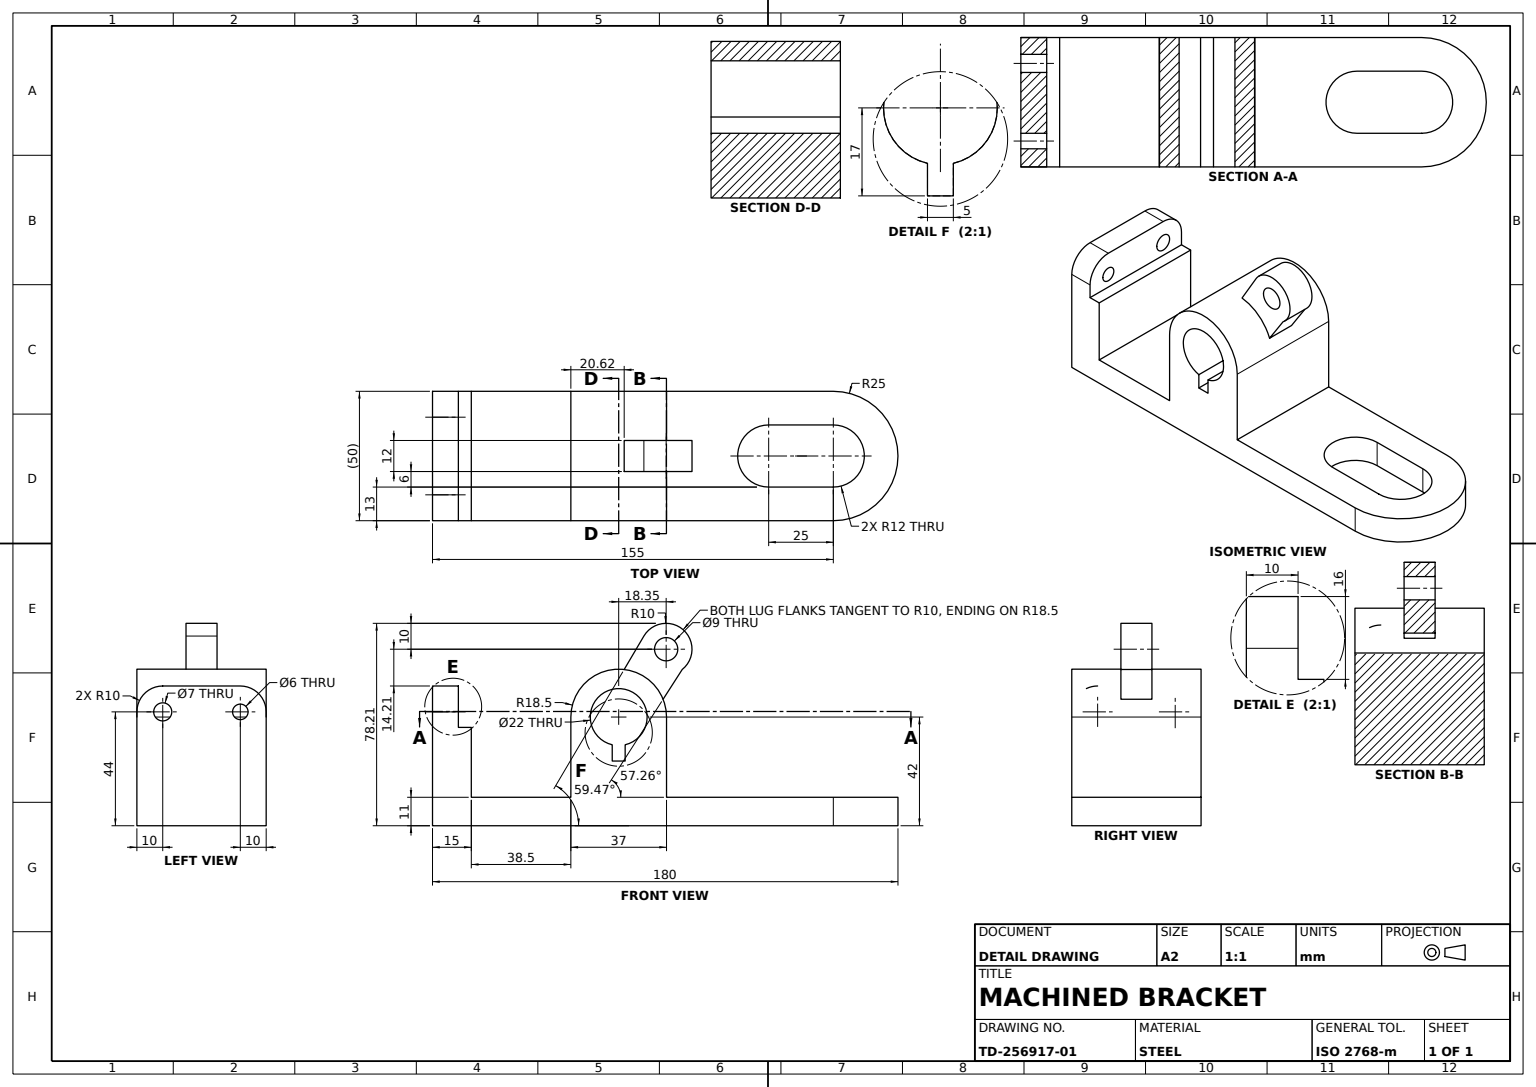
SolidWorks part; units mm, degrees
material "Plain Carbon Steel"
ref_plane "Front Plane" through (0, 0, 0) normal (0, 0, 1) x (1, 0, 0)
ref_plane "Top Plane" through (0, 0, 0) normal (0, 1, 0) x (1, 0, 0)
ref_plane "Right Plane" through (0, 0, 0) normal (1, 0, 0) x (0, 0, -1)
sketch "Base Plate Sketch" plane through (0, 0, 0) normal (0, 1, 0) x (1, 0, 0)
  line L0 (-77.5, 25) -> (-77.5, -25)
  line L2 (-77.5, 25) -> (77.5, 25)
  line L4 (77.5, -25) -> (-77.5, -25)
  arc A0 (77.5, -25) -> (77.5, 25) centre (77.5, 0) ccw
  dimension "D2" = 25
  dimension "D1" = 155
  dimension "D3" = 25
  dimension "D4" = 77.5
extrude "Base Plate 11mm" add sketch "Base Plate Sketch" along normal blind 11
sketch "Upright Block Sketch" plane through (0, 0, 25) normal (0, 0, 1) x (1, 0, 0)
  line L0 (-77.5, 0) -> (-5.5, 0)
  line L1 (-77.5, 0) -> (77.5, 0) construction
  line L2 (77.5, 11) -> (77.5, 0) construction
  line L3 (-24, 42) -> (-24, 11)
  line L4 (-77.5, 11) -> (77.5, 11) construction
  line L5 (13, 42) -> (13, 11)
  line L6 (-24, 11) -> (13, 11)
  arc A0 (13, 42) -> (-24, 42) centre (-5.5, 42) ccw
  line M7 (77.5, 11) -> (-77.5, 11)
  dimension "D1" = 18.5
  dimension "D2" = 83
  dimension "D3" = 42
extrude "Upright Block" add sketch "Upright Block Sketch" against normal blind 50 contours L5 A0 L3 M7
sketch "Channel Cut Sketch" plane through (0, 0, 25) normal (0, 0, 1) x (1, 0, 0)
  line L0 (77.5, 11) -> (77.5, 0) construction
  line L1 (-5.5, 25) -> (-8, 25)
  line L2 (-8, 25) -> (-8, 31.2879)
  line L3 (-5.5, 25) -> (-3, 25)
  line L4 (-3, 25) -> (-3, 31.2879)
  line L5 (-77.5, 0) -> (77.5, 0) construction
  arc A0 (-3, 31.2879) -> (-8, 31.2879) centre (-5.5, 42) ccw
  dimension "D1" = 11
  dimension "D2" = 80.5
  dimension "D3" = 25
extrude "Channel Cut" cut sketch "Channel Cut Sketch" against normal blind 50 contours A0 L2 L1 L3 L4
sketch "Front Wall Sketch" plane through (0, 0, 0) normal (0, 0, 1) x (1, 0, 0)
  line L1 (4.2411, 73.2933) -> (-3.3769, 60.3778)
  line L2 (19.0698, 60.379) -> (11.6741, 48.8774)
  line L3 (-3.3769, 60.3778) -> (11.6741, 48.8774)
  arc A0 (19.0698, 60.379) -> (4.2411, 73.2933) centre (12.8544, 68.2129) ccw
  arc A1 (13, 42) -> (-24, 42) centre (-5.5, 42) ccw construction
  dimension "D1" = 10
  dimension "D2" = 6.2154
  dimension "D3" = 7.3957
  dimension "D4" = 14.8287
  dimension "D5" = 22.4467
  dimension "D6" = 24.4159
extrude "Front Wall 12mm" add sketch "Front Wall Sketch" along normal mid plane 12
sketch "Wall Hole Sketch" plane through (0, 0, 6) normal (0, 0, 1) x (1, 0, 0)
  circle A0 centre (12.8544, 68.2129) radius 4.5
  dimension "D1" = 9
extrude "Wall Through Hole" cut sketch "Wall Hole Sketch" against normal blind 69
sketch "Bore Keyway Sketch" plane through (0, 11, 0) normal (0, 1, 0) x (1, 0, 0)
  line L0 (52.5, 12) -> (77.5, 12)
  line L1 (52.5, -12) -> (77.5, -12)
  line L2 (13, 25) -> (13, -25) construction
  arc A0 (77.5, -12) -> (77.5, 12) centre (77.5, 0) ccw
  arc A1 (52.5, 12) -> (52.5, -12) centre (52.5, 0) ccw
  dimension "D1" = 12
  dimension "D2" = 39.5
extrude "Bore Keyway Cut" cut sketch "Bore Keyway Sketch" against normal blind 69
sketch "Housing Pad Sketch" plane through (0, 11, 0) normal (0, 1, 0) x (1, 0, 0)
  line L0 (-77.5, -25) -> (-62.5, -25)
  line L1 (-77.5, -25) -> (-24, -25) construction
  line L2 (-62.5, -25) -> (-62.5, 25)
  line L3 (-24, 25) -> (-77.5, 25) construction
  line L4 (-62.5, 25) -> (-77.5, 25)
  line L5 (-77.5, 25) -> (-77.5, -25)
  line L6 (-24, 25) -> (-24, -25) construction
  dimension "D1" = 38.5
extrude "Housing Pad" add sketch "Housing Pad Sketch" along normal blind 27
sketch "Bore Housing Sketch" plane through (0, 0, 25) normal (0, 0, 1) x (1, 0, 0)
  line L0 (-77.5, 38) -> (-67.5, 38)
  line L1 (-77.5, 38) -> (-62.5, 38) construction
  line L2 (-67.5, 38) -> (-67.5, 54)
  line L3 (-67.5, 54) -> (-77.5, 54)
  line L4 (-77.5, 54) -> (-77.5, 38)
  line L5 (77.5, 11) -> (77.5, 0) construction
  point P7 (-67.5, 46)
  dimension "D1" = 8
  dimension "D2" = 145
extrude "Bore Housing" add sketch "Bore Housing Sketch" against normal blind 50
fillet "Housing Fillet R10 A" radius 10 1 edges at (-72.5, 54, 25)
fillet "Housing Fillet R10 B" radius 10 1 edges at (-72.5, 54, -25)
sketch "Cross Hole Sketch" plane through (-77.5, 0, 0) normal (-1, 0, 0) x (0, 0, 1)
  circle A0 centre (-15, 44) radius 3.5
  circle A1 centre (15, 44) radius 3
  dimension "D1" = 6
  dimension "D2" = 7
extrude "Housing Cross Hole" cut sketch "Cross Hole Sketch" against normal blind 40
